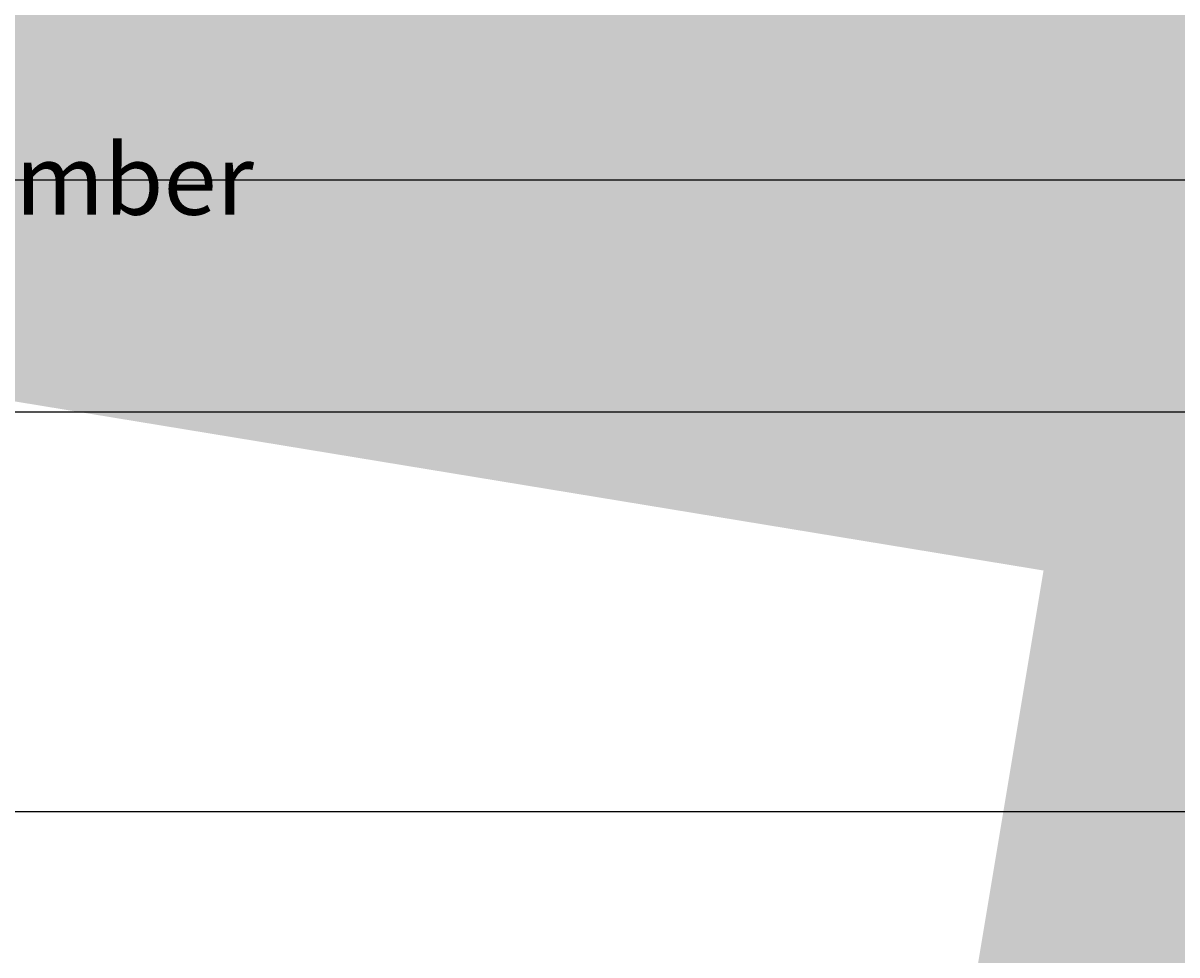
# Model space of a CAD drawing. Units: millimetres. Extents: x -22994 to 29398, y -19990 to 20176.
# Tile 56 of 135: x 247 to 296, y 25 to 65. Entities that reach past the tile are written whole.
import ezdxf
from ezdxf import colors
from ezdxf.entities.mleader import LeaderData, LeaderLine
from ezdxf.math import Vec2, Vec3

# ---------------------------------------------------------------- set-up
doc = ezdxf.new("R2010")
doc.units = ezdxf.units.MM
doc.header["$MEASUREMENT"] = 0
doc.layers.add('M-ANNO-TEXT', color=7, linetype='Continuous', lineweight=25)
doc.layers.add('M-DIMS', color=2, linetype='Continuous', lineweight=18)
doc.styles.get("Standard").update_dxf_attribs({"font": 'arial.ttf'})
doc.dimstyles.get("Standard").update_dxf_attribs({"dimtxt": 0.18, "dimasz": 10000, "dimexe": 0.18, "dimexo": 0.0625, "dimgap": 0.09, "dimtad": 0, "dimtih": 1, "dimtoh": 1, "dimdec": 0, "dimzin": 0, "dimdsep": 46, "dimtxsty": 'Standard', "dimcen": 0.09, "dimadec": 0, "dimazin": 0, "dimtfac": 1, "dimtdec": 0, "dimtofl": 0, "dimtmove": 0, "dimatfit": 3, "dimfxl": 1, "dimtolj": 1, "dimtzin": 0, "dimlwd": 30, "dimarcsym": 0})

# ---------------------------------------------------------------- blocks, each defined once
blk = doc.blocks.new('*D2')
at = {"layer": 'Defpoints', "color": 0, "transparency": 16777216}
for p in [(6.677, 10.271), (290.852, 10.271), (290.852, -5.079)]:
    blk.add_point(p, dxfattribs=at)
at = {"layer": 'M-DIMS', "color": 0, "lineweight": -2, "transparency": 16777216}
for p, q in [((6.677, 10.209), (6.677, -5.259)), ((290.852, 10.209), (290.852, -5.259))]:
    blk.add_line(p, q, dxfattribs=at)
at = {"layer": 'M-DIMS', "color": 0, "lineweight": 30, "transparency": 16777216}
for p, q in [((-9993.323, -5.079), (-19993.323, -5.079)), ((10290.852, -5.079), (20290.852, -5.079))]:
    blk.add_line(p, q, dxfattribs=at)
at = {"layer": 'M-DIMS', "color": 0, "transparency": 16777216}
for points in [[(-9993.323, 1661.588), (-9993.323, -1671.745), (6.677, -5.079)], [(10290.852, 1661.588), (10290.852, -1671.745), (290.852, -5.079)]]:
    blk.add_solid(points, dxfattribs=at)
at = {"layer": 'M-DIMS', "color": 0, "transparency": 16777216, "insert": (148.765, -5.079), "char_height": 0.18, "attachment_point": 5}
blk.add_mtext('\\A1;284.2', dxfattribs=at)
blk = doc.blocks.new('*D3')
at = {"layer": 'Defpoints', "color": 0, "transparency": 16777216}
for p in [(110.265, 204.165), (110.265, 176.366), (95.833, 127.967)]:
    blk.add_point(p, dxfattribs=at)
at = {"layer": 'M-DIMS', "color": 0, "lineweight": -2, "transparency": 16777216}
for p, q in [((95.833, 128.03), (95.833, 204.345)), ((110.265, 176.429), (110.265, 204.345))]:
    blk.add_line(p, q, dxfattribs=at)
at = {"layer": 'M-DIMS', "color": 0, "lineweight": 30, "transparency": 16777216}
for p, q in [((-9904.167, 204.165), (-19904.167, 204.165)), ((10110.265, 204.165), (20110.265, 204.165))]:
    blk.add_line(p, q, dxfattribs=at)
at = {"layer": 'M-DIMS', "color": 0, "transparency": 16777216}
for points in [[(-9904.167, 1870.832), (-9904.167, -1462.501), (95.833, 204.165)], [(10110.265, 1870.832), (10110.265, -1462.501), (110.265, 204.165)]]:
    blk.add_solid(points, dxfattribs=at)
at = {"layer": 'M-DIMS', "color": 0, "transparency": 16777216, "insert": (103.049, 204.165), "char_height": 0.18, "attachment_point": 5}
blk.add_mtext('\\A1;14.432', dxfattribs=at)
blk = doc.blocks.new('*D4')
at = {"layer": 'Defpoints', "color": 0, "transparency": 16777216}
for p in [(116.265, 204.165), (110.265, 176.366), (116.265, 176.366)]:
    blk.add_point(p, dxfattribs=at)
at = {"layer": 'M-DIMS', "color": 0, "lineweight": -2, "transparency": 16777216}
for p, q in [((110.265, 176.429), (110.265, 204.345)), ((116.265, 176.429), (116.265, 204.345))]:
    blk.add_line(p, q, dxfattribs=at)
at = {"layer": 'M-DIMS', "color": 0, "lineweight": 30, "transparency": 16777216}
for p, q in [((-9889.735, 204.165), (-19889.735, 204.165)), ((10116.265, 204.165), (20116.265, 204.165))]:
    blk.add_line(p, q, dxfattribs=at)
at = {"layer": 'M-DIMS', "color": 0, "transparency": 16777216}
for points in [[(-9889.735, 1870.832), (-9889.735, -1462.501), (110.265, 204.165)], [(10116.265, 1870.832), (10116.265, -1462.501), (116.265, 204.165)]]:
    blk.add_solid(points, dxfattribs=at)
at = {"layer": 'M-DIMS', "color": 0, "transparency": 16777216, "insert": (113.265, 204.165), "char_height": 0.18, "attachment_point": 5}
blk.add_mtext('\\A1;6', dxfattribs=at)
blk = doc.blocks.new('*D5')
at = {"layer": 'Defpoints', "color": 0, "transparency": 16777216}
for p in [(181.265, 204.165), (116.265, 176.366), (181.265, 176.366)]:
    blk.add_point(p, dxfattribs=at)
at = {"layer": 'M-DIMS', "color": 0, "lineweight": -2, "transparency": 16777216}
for p, q in [((116.265, 176.429), (116.265, 204.345)), ((181.265, 176.429), (181.265, 204.345))]:
    blk.add_line(p, q, dxfattribs=at)
at = {"layer": 'M-DIMS', "color": 0, "lineweight": 30, "transparency": 16777216}
for p, q in [((-9883.735, 204.165), (-19883.735, 204.165)), ((10181.265, 204.165), (20181.265, 204.165))]:
    blk.add_line(p, q, dxfattribs=at)
at = {"layer": 'M-DIMS', "color": 0, "transparency": 16777216}
for points in [[(-9883.735, 1870.832), (-9883.735, -1462.501), (116.265, 204.165)], [(10181.265, 1870.832), (10181.265, -1462.501), (181.265, 204.165)]]:
    blk.add_solid(points, dxfattribs=at)
at = {"layer": 'M-DIMS', "color": 0, "transparency": 16777216, "insert": (148.765, 204.165), "char_height": 0.18, "attachment_point": 5}
blk.add_mtext('\\A1;65', dxfattribs=at)
blk = doc.blocks.new('*D6')
at = {"layer": 'Defpoints', "color": 0, "transparency": 16777216}
for p in [(187.265, 204.165), (181.265, 176.366), (187.265, 176.366)]:
    blk.add_point(p, dxfattribs=at)
at = {"layer": 'M-DIMS', "color": 0, "lineweight": -2, "transparency": 16777216}
for p, q in [((181.265, 176.429), (181.265, 204.345)), ((187.265, 176.429), (187.265, 204.345))]:
    blk.add_line(p, q, dxfattribs=at)
at = {"layer": 'M-DIMS', "color": 0, "lineweight": 30, "transparency": 16777216}
for p, q in [((-9818.735, 204.165), (-19818.735, 204.165)), ((10187.265, 204.165), (20187.265, 204.165))]:
    blk.add_line(p, q, dxfattribs=at)
at = {"layer": 'M-DIMS', "color": 0, "transparency": 16777216}
for points in [[(-9818.735, 1870.832), (-9818.735, -1462.501), (181.265, 204.165)], [(10187.265, 1870.832), (10187.265, -1462.501), (187.265, 204.165)]]:
    blk.add_solid(points, dxfattribs=at)
at = {"layer": 'M-DIMS', "color": 0, "transparency": 16777216, "insert": (184.265, 204.165), "char_height": 0.18, "attachment_point": 5}
blk.add_mtext('\\A1;6', dxfattribs=at)
blk = doc.blocks.new('*D7')
at = {"layer": 'Defpoints', "color": 0, "transparency": 16777216}
for p in [(201.697, 204.165), (187.265, 176.366), (201.697, 127.967)]:
    blk.add_point(p, dxfattribs=at)
at = {"layer": 'M-DIMS', "color": 0, "lineweight": -2, "transparency": 16777216}
for p, q in [((187.265, 176.429), (187.265, 204.345)), ((201.697, 128.03), (201.697, 204.345))]:
    blk.add_line(p, q, dxfattribs=at)
at = {"layer": 'M-DIMS', "color": 0, "lineweight": 30, "transparency": 16777216}
for p, q in [((-9812.735, 204.165), (-19812.735, 204.165)), ((10201.697, 204.165), (20201.697, 204.165))]:
    blk.add_line(p, q, dxfattribs=at)
at = {"layer": 'M-DIMS', "color": 0, "transparency": 16777216}
for points in [[(-9812.735, 1870.832), (-9812.735, -1462.501), (187.265, 204.165)], [(10201.697, 1870.832), (10201.697, -1462.501), (201.697, 204.165)]]:
    blk.add_solid(points, dxfattribs=at)
at = {"layer": 'M-DIMS', "color": 0, "transparency": 16777216, "insert": (194.481, 204.165), "char_height": 0.18, "attachment_point": 5}
blk.add_mtext('\\A1;14.432', dxfattribs=at)
blk = doc.blocks.new('*D8')
at = {"layer": 'Defpoints', "color": 0, "transparency": 16777216}
for p in [(227.648, 204.165), (227.648, 146.73), (201.697, 127.967)]:
    blk.add_point(p, dxfattribs=at)
at = {"layer": 'M-DIMS', "color": 0, "lineweight": -2, "transparency": 16777216}
for p, q in [((201.697, 128.03), (201.697, 204.345)), ((227.648, 146.792), (227.648, 204.345))]:
    blk.add_line(p, q, dxfattribs=at)
at = {"layer": 'M-DIMS', "color": 0, "lineweight": 30, "transparency": 16777216}
for p, q in [((-9798.303, 204.165), (-19798.303, 204.165)), ((10227.648, 204.165), (20227.648, 204.165))]:
    blk.add_line(p, q, dxfattribs=at)
at = {"layer": 'M-DIMS', "color": 0, "transparency": 16777216}
for points in [[(-9798.303, 1870.832), (-9798.303, -1462.501), (201.697, 204.165)], [(10227.648, 1870.832), (10227.648, -1462.501), (227.648, 204.165)]]:
    blk.add_solid(points, dxfattribs=at)
at = {"layer": 'M-DIMS', "color": 0, "transparency": 16777216, "insert": (214.673, 204.165), "char_height": 0.18, "attachment_point": 5}
blk.add_mtext('\\A1;25.95', dxfattribs=at)
blk = doc.blocks.new('*D9')
at = {"layer": 'Defpoints', "color": 0, "transparency": 16777216}
for p in [(187.265, 176.366), (306.202, 176.366), (290.852, 10.271)]:
    blk.add_point(p, dxfattribs=at)
at = {"layer": 'M-DIMS', "color": 0, "lineweight": 30, "transparency": 16777216}
for p, q in [((306.202, 10176.366), (306.202, 20176.366)), ((306.202, -9989.729), (306.202, -19989.729))]:
    blk.add_line(p, q, dxfattribs=at)
at = {"layer": 'M-DIMS', "color": 0, "lineweight": -2, "transparency": 16777216}
for p, q in [((187.327, 176.366), (306.382, 176.366)), ((290.915, 10.271), (306.382, 10.271))]:
    blk.add_line(p, q, dxfattribs=at)
at = {"layer": 'M-DIMS', "color": 0, "transparency": 16777216}
for points in [[(-1360.465, 10176.366), (1972.869, 10176.366), (306.202, 176.366)], [(-1360.465, -9989.729), (1972.869, -9989.729), (306.202, 10.271)]]:
    blk.add_solid(points, dxfattribs=at)
at = {"layer": 'M-DIMS', "color": 0, "transparency": 16777216, "insert": (306.202, 93.319), "char_height": 0.18, "attachment_point": 5}
blk.add_mtext('\\A1;166.1', dxfattribs=at)
blk = doc.blocks.new('*D10')
at = {"layer": 'Defpoints', "color": 0, "transparency": 16777216}
for p in [(125.65, 136.071), (133.346, 136.071), (133.346, -5.079)]:
    blk.add_point(p, dxfattribs=at)
at = {"layer": 'M-DIMS', "color": 0, "lineweight": -2, "transparency": 16777216}
for p, q in [((125.65, 136.009), (125.65, -5.259)), ((133.346, 136.009), (133.346, -5.259))]:
    blk.add_line(p, q, dxfattribs=at)
at = {"layer": 'M-DIMS', "color": 0, "lineweight": 30, "transparency": 16777216}
for p, q in [((-9874.35, -5.079), (-19874.35, -5.079)), ((10133.346, -5.079), (20133.346, -5.079))]:
    blk.add_line(p, q, dxfattribs=at)
at = {"layer": 'M-DIMS', "color": 0, "transparency": 16777216}
for points in [[(-9874.35, 1661.588), (-9874.35, -1671.745), (125.65, -5.079)], [(10133.346, 1661.588), (10133.346, -1671.745), (133.346, -5.079)]]:
    blk.add_solid(points, dxfattribs=at)
at = {"layer": 'M-DIMS', "color": 0, "transparency": 16777216, "insert": (129.498, -5.079), "char_height": 0.18, "attachment_point": 5}
blk.add_mtext('\\A1;7.696', dxfattribs=at)
blk = doc.blocks.new('*D11')
at = {"layer": 'Defpoints', "color": 0, "transparency": 16777216}
for p in [(133.346, 136.071), (135.65, 136.071), (135.65, -5.079)]:
    blk.add_point(p, dxfattribs=at)
at = {"layer": 'M-DIMS', "color": 0, "lineweight": -2, "transparency": 16777216}
for p, q in [((133.346, 136.009), (133.346, -5.259)), ((135.65, 136.009), (135.65, -5.259))]:
    blk.add_line(p, q, dxfattribs=at)
at = {"layer": 'M-DIMS', "color": 0, "lineweight": 30, "transparency": 16777216}
for p, q in [((-9866.654, -5.079), (-19866.654, -5.079)), ((10135.65, -5.079), (20135.65, -5.079))]:
    blk.add_line(p, q, dxfattribs=at)
at = {"layer": 'M-DIMS', "color": 0, "transparency": 16777216}
for points in [[(-9866.654, 1661.588), (-9866.654, -1671.745), (133.346, -5.079)], [(10135.65, 1661.588), (10135.65, -1671.745), (135.65, -5.079)]]:
    blk.add_solid(points, dxfattribs=at)
at = {"layer": 'M-DIMS', "color": 0, "transparency": 16777216, "insert": (134.498, -5.079), "char_height": 0.18, "attachment_point": 5}
blk.add_mtext('\\A1;2.304', dxfattribs=at)
blk = doc.blocks.new('*D12')
at = {"layer": 'Defpoints', "color": 0, "transparency": 16777216}
for p in [(135.65, 136.071), (145.65, 136.071), (145.65, -5.079)]:
    blk.add_point(p, dxfattribs=at)
at = {"layer": 'M-DIMS', "color": 0, "lineweight": -2, "transparency": 16777216}
for p, q in [((135.65, 136.009), (135.65, -5.259)), ((145.65, 136.009), (145.65, -5.259))]:
    blk.add_line(p, q, dxfattribs=at)
at = {"layer": 'M-DIMS', "color": 0, "lineweight": 30, "transparency": 16777216}
for p, q in [((-9864.35, -5.079), (-19864.35, -5.079)), ((10145.65, -5.079), (20145.65, -5.079))]:
    blk.add_line(p, q, dxfattribs=at)
at = {"layer": 'M-DIMS', "color": 0, "transparency": 16777216}
for points in [[(-9864.35, 1661.588), (-9864.35, -1671.745), (135.65, -5.079)], [(10145.65, 1661.588), (10145.65, -1671.745), (145.65, -5.079)]]:
    blk.add_solid(points, dxfattribs=at)
at = {"layer": 'M-DIMS', "color": 0, "transparency": 16777216, "insert": (140.65, -5.079), "char_height": 0.18, "attachment_point": 5}
blk.add_mtext('\\A1;10', dxfattribs=at)
blk = doc.blocks.new('*D13')
at = {"layer": 'Defpoints', "color": 0, "transparency": 16777216}
for p in [(145.65, 136.071), (155.65, 136.071), (155.65, -5.079)]:
    blk.add_point(p, dxfattribs=at)
at = {"layer": 'M-DIMS', "color": 0, "lineweight": -2, "transparency": 16777216}
for p, q in [((145.65, 136.009), (145.65, -5.259)), ((155.65, 136.009), (155.65, -5.259))]:
    blk.add_line(p, q, dxfattribs=at)
at = {"layer": 'M-DIMS', "color": 0, "lineweight": 30, "transparency": 16777216}
for p, q in [((-9854.35, -5.079), (-19854.35, -5.079)), ((10155.65, -5.079), (20155.65, -5.079))]:
    blk.add_line(p, q, dxfattribs=at)
at = {"layer": 'M-DIMS', "color": 0, "transparency": 16777216}
for points in [[(-9854.35, 1661.588), (-9854.35, -1671.745), (145.65, -5.079)], [(10155.65, 1661.588), (10155.65, -1671.745), (155.65, -5.079)]]:
    blk.add_solid(points, dxfattribs=at)
at = {"layer": 'M-DIMS', "color": 0, "transparency": 16777216, "insert": (150.65, -5.079), "char_height": 0.18, "attachment_point": 5}
blk.add_mtext('\\A1;10', dxfattribs=at)
blk = doc.blocks.new('*D14')
at = {"layer": 'Defpoints', "color": 0, "transparency": 16777216}
for p in [(155.65, 136.071), (165.65, 136.071), (165.65, -5.079)]:
    blk.add_point(p, dxfattribs=at)
at = {"layer": 'M-DIMS', "color": 0, "lineweight": -2, "transparency": 16777216}
for p, q in [((155.65, 136.009), (155.65, -5.259)), ((165.65, 136.009), (165.65, -5.259))]:
    blk.add_line(p, q, dxfattribs=at)
at = {"layer": 'M-DIMS', "color": 0, "lineweight": 30, "transparency": 16777216}
for p, q in [((-9844.35, -5.079), (-19844.35, -5.079)), ((10165.65, -5.079), (20165.65, -5.079))]:
    blk.add_line(p, q, dxfattribs=at)
at = {"layer": 'M-DIMS', "color": 0, "transparency": 16777216}
for points in [[(-9844.35, 1661.588), (-9844.35, -1671.745), (155.65, -5.079)], [(10165.65, 1661.588), (10165.65, -1671.745), (165.65, -5.079)]]:
    blk.add_solid(points, dxfattribs=at)
at = {"layer": 'M-DIMS', "color": 0, "transparency": 16777216, "insert": (160.65, -5.079), "char_height": 0.18, "attachment_point": 5}
blk.add_mtext('\\A1;10', dxfattribs=at)
blk = doc.blocks.new('*D15')
at = {"layer": 'Defpoints', "color": 0, "transparency": 16777216}
for p in [(173.346, 154.788), (173.346, 136.071), (306.202, 136.071)]:
    blk.add_point(p, dxfattribs=at)
at = {"layer": 'M-DIMS', "color": 0, "lineweight": 30, "transparency": 16777216}
for p, q in [((306.202, 10154.788), (306.202, 20154.788)), ((306.202, -9863.929), (306.202, -19863.929))]:
    blk.add_line(p, q, dxfattribs=at)
at = {"layer": 'M-DIMS', "color": 0, "lineweight": -2, "transparency": 16777216}
for p, q in [((173.408, 154.788), (306.382, 154.788)), ((173.408, 136.071), (306.382, 136.071))]:
    blk.add_line(p, q, dxfattribs=at)
at = {"layer": 'M-DIMS', "color": 0, "transparency": 16777216}
for points in [[(-1360.465, 10154.788), (1972.869, 10154.788), (306.202, 154.788)], [(-1360.465, -9863.929), (1972.869, -9863.929), (306.202, 136.071)]]:
    blk.add_solid(points, dxfattribs=at)
at = {"layer": 'M-DIMS', "color": 0, "transparency": 16777216, "insert": (306.202, 145.43), "char_height": 0.18, "attachment_point": 5}
blk.add_mtext('\\A1;18.717', dxfattribs=at)
blk = doc.blocks.new('*D16')
at = {"layer": 'Defpoints', "color": 0, "transparency": 16777216}
for p in [(120.17, 204.165), (110.466, 48.035), (120.17, 48.035)]:
    blk.add_point(p, dxfattribs=at)
at = {"layer": 'M-DIMS', "color": 0, "lineweight": -2, "transparency": 16777216}
for p, q in [((110.466, 48.097), (110.466, 204.345)), ((120.17, 48.097), (120.17, 204.345))]:
    blk.add_line(p, q, dxfattribs=at)
at = {"layer": 'M-DIMS', "color": 0, "lineweight": 30, "transparency": 16777216}
for p, q in [((-9889.534, 204.165), (-19889.534, 204.165)), ((10120.17, 204.165), (20120.17, 204.165))]:
    blk.add_line(p, q, dxfattribs=at)
at = {"layer": 'M-DIMS', "color": 0, "transparency": 16777216}
for points in [[(-9889.534, 1870.832), (-9889.534, -1462.501), (110.466, 204.165)], [(10120.17, 1870.832), (10120.17, -1462.501), (120.17, 204.165)]]:
    blk.add_solid(points, dxfattribs=at)
at = {"layer": 'M-DIMS', "color": 0, "transparency": 16777216, "insert": (115.318, 204.165), "char_height": 0.18, "attachment_point": 5}
blk.add_mtext('\\A1;9.704', dxfattribs=at)
blk = doc.blocks.new('*D17')
at = {"layer": 'Defpoints', "color": 0, "transparency": 16777216}
for p in [(126.17, 204.165), (120.17, 48.035), (126.17, 48.035)]:
    blk.add_point(p, dxfattribs=at)
at = {"layer": 'M-DIMS', "color": 0, "lineweight": -2, "transparency": 16777216}
for p, q in [((120.17, 48.097), (120.17, 204.345)), ((126.17, 48.097), (126.17, 204.345))]:
    blk.add_line(p, q, dxfattribs=at)
at = {"layer": 'M-DIMS', "color": 0, "lineweight": 30, "transparency": 16777216}
for p, q in [((-9879.83, 204.165), (-19879.83, 204.165)), ((10126.17, 204.165), (20126.17, 204.165))]:
    blk.add_line(p, q, dxfattribs=at)
at = {"layer": 'M-DIMS', "color": 0, "transparency": 16777216}
for points in [[(-9879.83, 1870.832), (-9879.83, -1462.501), (120.17, 204.165)], [(10126.17, 1870.832), (10126.17, -1462.501), (126.17, 204.165)]]:
    blk.add_solid(points, dxfattribs=at)
at = {"layer": 'M-DIMS', "color": 0, "transparency": 16777216, "insert": (123.17, 204.165), "char_height": 0.18, "attachment_point": 5}
blk.add_mtext('\\A1;6', dxfattribs=at)
blk = doc.blocks.new('*D18')
at = {"layer": 'Defpoints', "color": 0, "transparency": 16777216}
for p in [(132.17, 204.165), (126.17, 48.035), (132.17, 48.035)]:
    blk.add_point(p, dxfattribs=at)
at = {"layer": 'M-DIMS', "color": 0, "lineweight": -2, "transparency": 16777216}
for p, q in [((126.17, 48.097), (126.17, 204.345)), ((132.17, 48.097), (132.17, 204.345))]:
    blk.add_line(p, q, dxfattribs=at)
at = {"layer": 'M-DIMS', "color": 0, "lineweight": 30, "transparency": 16777216}
for p, q in [((-9873.83, 204.165), (-19873.83, 204.165)), ((10132.17, 204.165), (20132.17, 204.165))]:
    blk.add_line(p, q, dxfattribs=at)
at = {"layer": 'M-DIMS', "color": 0, "transparency": 16777216}
for points in [[(-9873.83, 1870.832), (-9873.83, -1462.501), (126.17, 204.165)], [(10132.17, 1870.832), (10132.17, -1462.501), (132.17, 204.165)]]:
    blk.add_solid(points, dxfattribs=at)
at = {"layer": 'M-DIMS', "color": 0, "transparency": 16777216, "insert": (129.17, 204.165), "char_height": 0.18, "attachment_point": 5}
blk.add_mtext('\\A1;6', dxfattribs=at)
blk = doc.blocks.new('*D19')
at = {"layer": 'Defpoints', "color": 0, "transparency": 16777216}
for p in [(138.17, 204.165), (132.17, 48.035), (138.17, 48.035)]:
    blk.add_point(p, dxfattribs=at)
at = {"layer": 'M-DIMS', "color": 0, "lineweight": -2, "transparency": 16777216}
for p, q in [((132.17, 48.097), (132.17, 204.345)), ((138.17, 48.097), (138.17, 204.345))]:
    blk.add_line(p, q, dxfattribs=at)
at = {"layer": 'M-DIMS', "color": 0, "lineweight": 30, "transparency": 16777216}
for p, q in [((-9867.83, 204.165), (-19867.83, 204.165)), ((10138.17, 204.165), (20138.17, 204.165))]:
    blk.add_line(p, q, dxfattribs=at)
at = {"layer": 'M-DIMS', "color": 0, "transparency": 16777216}
for points in [[(-9867.83, 1870.832), (-9867.83, -1462.501), (132.17, 204.165)], [(10138.17, 1870.832), (10138.17, -1462.501), (138.17, 204.165)]]:
    blk.add_solid(points, dxfattribs=at)
at = {"layer": 'M-DIMS', "color": 0, "transparency": 16777216, "insert": (135.17, 204.165), "char_height": 0.18, "attachment_point": 5}
blk.add_mtext('\\A1;6', dxfattribs=at)
blk = doc.blocks.new('*D20')
at = {"layer": 'Defpoints', "color": 0, "transparency": 16777216}
for p in [(144.17, 204.165), (138.17, 48.035), (144.17, 48.035)]:
    blk.add_point(p, dxfattribs=at)
at = {"layer": 'M-DIMS', "color": 0, "lineweight": -2, "transparency": 16777216}
for p, q in [((138.17, 48.097), (138.17, 204.345)), ((144.17, 48.097), (144.17, 204.345))]:
    blk.add_line(p, q, dxfattribs=at)
at = {"layer": 'M-DIMS', "color": 0, "lineweight": 30, "transparency": 16777216}
for p, q in [((-9861.83, 204.165), (-19861.83, 204.165)), ((10144.17, 204.165), (20144.17, 204.165))]:
    blk.add_line(p, q, dxfattribs=at)
at = {"layer": 'M-DIMS', "color": 0, "transparency": 16777216}
for points in [[(-9861.83, 1870.832), (-9861.83, -1462.501), (138.17, 204.165)], [(10144.17, 1870.832), (10144.17, -1462.501), (144.17, 204.165)]]:
    blk.add_solid(points, dxfattribs=at)
at = {"layer": 'M-DIMS', "color": 0, "transparency": 16777216, "insert": (141.17, 204.165), "char_height": 0.18, "attachment_point": 5}
blk.add_mtext('\\A1;6', dxfattribs=at)
blk = doc.blocks.new('*D21')
at = {"layer": 'Defpoints', "color": 0, "transparency": 16777216}
for p in [(149.116, 204.165), (144.17, 48.035), (149.116, 48.035)]:
    blk.add_point(p, dxfattribs=at)
at = {"layer": 'M-DIMS', "color": 0, "lineweight": -2, "transparency": 16777216}
for p, q in [((144.17, 48.097), (144.17, 204.345)), ((149.116, 48.097), (149.116, 204.345))]:
    blk.add_line(p, q, dxfattribs=at)
at = {"layer": 'M-DIMS', "color": 0, "lineweight": 30, "transparency": 16777216}
for p, q in [((-9855.83, 204.165), (-19855.83, 204.165)), ((10149.116, 204.165), (20149.116, 204.165))]:
    blk.add_line(p, q, dxfattribs=at)
at = {"layer": 'M-DIMS', "color": 0, "transparency": 16777216}
for points in [[(-9855.83, 1870.832), (-9855.83, -1462.501), (144.17, 204.165)], [(10149.116, 1870.832), (10149.116, -1462.501), (149.116, 204.165)]]:
    blk.add_solid(points, dxfattribs=at)
at = {"layer": 'M-DIMS', "color": 0, "transparency": 16777216, "insert": (146.643, 204.165), "char_height": 0.18, "attachment_point": 5}
blk.add_mtext('\\A1;4.945', dxfattribs=at)
blk = doc.blocks.new('*D22')
at = {"layer": 'Defpoints', "color": 0, "transparency": 16777216}
for p in [(149.116, 30.99), (155.116, 30.99), (155.116, -5.079)]:
    blk.add_point(p, dxfattribs=at)
at = {"layer": 'M-DIMS', "color": 0, "lineweight": -2, "transparency": 16777216}
for p, q in [((149.116, 30.927), (149.116, -5.259)), ((155.116, 30.927), (155.116, -5.259))]:
    blk.add_line(p, q, dxfattribs=at)
at = {"layer": 'M-DIMS', "color": 0, "lineweight": 30, "transparency": 16777216}
for p, q in [((-9850.884, -5.079), (-19850.884, -5.079)), ((10155.116, -5.079), (20155.116, -5.079))]:
    blk.add_line(p, q, dxfattribs=at)
at = {"layer": 'M-DIMS', "color": 0, "transparency": 16777216}
for points in [[(-9850.884, 1661.588), (-9850.884, -1671.745), (149.116, -5.079)], [(10155.116, 1661.588), (10155.116, -1671.745), (155.116, -5.079)]]:
    blk.add_solid(points, dxfattribs=at)
at = {"layer": 'M-DIMS', "color": 0, "transparency": 16777216, "insert": (152.116, -5.079), "char_height": 0.18, "attachment_point": 5}
blk.add_mtext('\\A1;6', dxfattribs=at)
blk = doc.blocks.new('*D23')
at = {"layer": 'Defpoints', "color": 0, "transparency": 16777216}
for p in [(155.116, 30.99), (161.116, 30.99), (161.116, -5.079)]:
    blk.add_point(p, dxfattribs=at)
at = {"layer": 'M-DIMS', "color": 0, "lineweight": -2, "transparency": 16777216}
for p, q in [((155.116, 30.927), (155.116, -5.259)), ((161.116, 30.927), (161.116, -5.259))]:
    blk.add_line(p, q, dxfattribs=at)
at = {"layer": 'M-DIMS', "color": 0, "lineweight": 30, "transparency": 16777216}
for p, q in [((-9844.884, -5.079), (-19844.884, -5.079)), ((10161.116, -5.079), (20161.116, -5.079))]:
    blk.add_line(p, q, dxfattribs=at)
at = {"layer": 'M-DIMS', "color": 0, "transparency": 16777216}
for points in [[(-9844.884, 1661.588), (-9844.884, -1671.745), (155.116, -5.079)], [(10161.116, 1661.588), (10161.116, -1671.745), (161.116, -5.079)]]:
    blk.add_solid(points, dxfattribs=at)
at = {"layer": 'M-DIMS', "color": 0, "transparency": 16777216, "insert": (158.116, -5.079), "char_height": 0.18, "attachment_point": 5}
blk.add_mtext('\\A1;6', dxfattribs=at)
blk = doc.blocks.new('*D24')
at = {"layer": 'Defpoints', "color": 0, "transparency": 16777216}
for p in [(161.116, 30.99), (166.439, 30.99), (166.439, -5.079)]:
    blk.add_point(p, dxfattribs=at)
at = {"layer": 'M-DIMS', "color": 0, "lineweight": -2, "transparency": 16777216}
for p, q in [((161.116, 30.927), (161.116, -5.259)), ((166.439, 30.927), (166.439, -5.259))]:
    blk.add_line(p, q, dxfattribs=at)
at = {"layer": 'M-DIMS', "color": 0, "lineweight": 30, "transparency": 16777216}
for p, q in [((-9838.884, -5.079), (-19838.884, -5.079)), ((10166.439, -5.079), (20166.439, -5.079))]:
    blk.add_line(p, q, dxfattribs=at)
at = {"layer": 'M-DIMS', "color": 0, "transparency": 16777216}
for points in [[(-9838.884, 1661.588), (-9838.884, -1671.745), (161.116, -5.079)], [(10166.439, 1661.588), (10166.439, -1671.745), (166.439, -5.079)]]:
    blk.add_solid(points, dxfattribs=at)
at = {"layer": 'M-DIMS', "color": 0, "transparency": 16777216, "insert": (163.777, -5.079), "char_height": 0.18, "attachment_point": 5}
blk.add_mtext('\\A1;5.323', dxfattribs=at)
blk = doc.blocks.new('*D25')
at = {"layer": 'Defpoints', "color": 0, "transparency": 16777216}
for p in [(166.439, 30.99), (172.439, 30.99), (172.439, -5.079)]:
    blk.add_point(p, dxfattribs=at)
at = {"layer": 'M-DIMS', "color": 0, "lineweight": -2, "transparency": 16777216}
for p, q in [((166.439, 30.927), (166.439, -5.259)), ((172.439, 30.927), (172.439, -5.259))]:
    blk.add_line(p, q, dxfattribs=at)
at = {"layer": 'M-DIMS', "color": 0, "lineweight": 30, "transparency": 16777216}
for p, q in [((-9833.561, -5.079), (-19833.561, -5.079)), ((10172.439, -5.079), (20172.439, -5.079))]:
    blk.add_line(p, q, dxfattribs=at)
at = {"layer": 'M-DIMS', "color": 0, "transparency": 16777216}
for points in [[(-9833.561, 1661.588), (-9833.561, -1671.745), (166.439, -5.079)], [(10172.439, 1661.588), (10172.439, -1671.745), (172.439, -5.079)]]:
    blk.add_solid(points, dxfattribs=at)
at = {"layer": 'M-DIMS', "color": 0, "transparency": 16777216, "insert": (169.439, -5.079), "char_height": 0.18, "attachment_point": 5}
blk.add_mtext('\\A1;6', dxfattribs=at)
blk = doc.blocks.new('*D26')
at = {"layer": 'Defpoints', "color": 0, "transparency": 16777216}
for p in [(172.439, 30.99), (178.439, 30.99), (178.439, -5.079)]:
    blk.add_point(p, dxfattribs=at)
at = {"layer": 'M-DIMS', "color": 0, "lineweight": -2, "transparency": 16777216}
for p, q in [((172.439, 30.927), (172.439, -5.259)), ((178.439, 30.927), (178.439, -5.259))]:
    blk.add_line(p, q, dxfattribs=at)
at = {"layer": 'M-DIMS', "color": 0, "lineweight": 30, "transparency": 16777216}
for p, q in [((-9827.561, -5.079), (-19827.561, -5.079)), ((10178.439, -5.079), (20178.439, -5.079))]:
    blk.add_line(p, q, dxfattribs=at)
at = {"layer": 'M-DIMS', "color": 0, "transparency": 16777216}
for points in [[(-9827.561, 1661.588), (-9827.561, -1671.745), (172.439, -5.079)], [(10178.439, 1661.588), (10178.439, -1671.745), (178.439, -5.079)]]:
    blk.add_solid(points, dxfattribs=at)
at = {"layer": 'M-DIMS', "color": 0, "transparency": 16777216, "insert": (175.439, -5.079), "char_height": 0.18, "attachment_point": 5}
blk.add_mtext('\\A1;6', dxfattribs=at)
blk = doc.blocks.new('*D27')
at = {"layer": 'Defpoints', "color": 0, "transparency": 16777216}
for p in [(178.439, 30.99), (188.117, 30.99), (188.117, -5.079)]:
    blk.add_point(p, dxfattribs=at)
at = {"layer": 'M-DIMS', "color": 0, "lineweight": -2, "transparency": 16777216}
for p, q in [((178.439, 30.927), (178.439, -5.259)), ((188.117, 30.927), (188.117, -5.259))]:
    blk.add_line(p, q, dxfattribs=at)
at = {"layer": 'M-DIMS', "color": 0, "lineweight": 30, "transparency": 16777216}
for p, q in [((-9821.561, -5.079), (-19821.561, -5.079)), ((10188.117, -5.079), (20188.117, -5.079))]:
    blk.add_line(p, q, dxfattribs=at)
at = {"layer": 'M-DIMS', "color": 0, "transparency": 16777216}
for points in [[(-9821.561, 1661.588), (-9821.561, -1671.745), (178.439, -5.079)], [(10188.117, 1661.588), (10188.117, -1671.745), (188.117, -5.079)]]:
    blk.add_solid(points, dxfattribs=at)
at = {"layer": 'M-DIMS', "color": 0, "transparency": 16777216, "insert": (183.278, -5.079), "char_height": 0.18, "attachment_point": 5}
blk.add_mtext('\\A1;9.679', dxfattribs=at)
blk = doc.blocks.new('*D28')
at = {"layer": 'Defpoints', "color": 0, "transparency": 16777216}
for p in [(188.117, 48.035), (306.202, 48.035), (188.117, 30.99)]:
    blk.add_point(p, dxfattribs=at)
at = {"layer": 'M-DIMS', "color": 0, "lineweight": 30, "transparency": 16777216}
for p, q in [((306.202, 10048.035), (306.202, 20048.035)), ((306.202, -9969.01), (306.202, -19969.01))]:
    blk.add_line(p, q, dxfattribs=at)
at = {"layer": 'M-DIMS', "color": 0, "lineweight": -2, "transparency": 16777216}
for p, q in [((188.18, 48.035), (306.382, 48.035)), ((188.18, 30.99), (306.382, 30.99))]:
    blk.add_line(p, q, dxfattribs=at)
at = {"layer": 'M-DIMS', "color": 0, "transparency": 16777216}
for points in [[(-1360.465, 10048.035), (1972.869, 10048.035), (306.202, 48.035)], [(-1360.465, -9969.01), (1972.869, -9969.01), (306.202, 30.99)]]:
    blk.add_solid(points, dxfattribs=at)
at = {"layer": 'M-DIMS', "color": 0, "transparency": 16777216, "insert": (306.202, 39.512), "char_height": 0.18, "attachment_point": 5}
blk.add_mtext('\\A1;17.045', dxfattribs=at)
blk = doc.blocks.new('*D29')
at = {"layer": 'Defpoints', "color": 0, "transparency": 16777216}
for p in [(36.801, 80.045), (64.03, 80.045)]:
    blk.add_point(p, dxfattribs=at)
at = {"layer": 'M-DIMS', "color": 0, "lineweight": -2, "transparency": 16777216}
for p, q in [((50.325, 80.045), (50.505, 80.045)), ((50.415, 79.955), (50.415, 80.135))]:
    blk.add_line(p, q, dxfattribs=at)
at = {"layer": 'M-DIMS', "color": 0, "lineweight": 30, "transparency": 16777216}
blk.add_line((20064.03, 80.03), (10064.03, 80.038), dxfattribs=at)
at = {"layer": 'M-DIMS', "color": 0, "transparency": 16777216}
blk.add_solid([(10064.031, 1746.704), (10064.028, -1586.629), (64.03, 80.045)], dxfattribs=at)
at = {"layer": 'M-DIMS', "color": 0, "transparency": 16777216, "insert": (20064.521, 80.03), "char_height": 0.18, "attachment_point": 5}
blk.add_mtext('\\A1;∅27.23', dxfattribs=at)
blk = doc.blocks.new('*D30')
at = {"layer": 'Defpoints', "color": 0, "transparency": 16777216}
for p in [(216.315, 146.729), (238.982, 146.73)]:
    blk.add_point(p, dxfattribs=at)
at = {"layer": 'M-DIMS', "color": 0, "lineweight": 30, "transparency": 16777216}
blk.add_line((20238.982, 147.496), (10238.982, 147.113), dxfattribs=at)
at = {"layer": 'M-DIMS', "color": 0, "lineweight": -2, "transparency": 16777216}
for p, q in [((227.558, 146.73), (227.738, 146.73)), ((227.648, 146.64), (227.648, 146.82))]:
    blk.add_line(p, q, dxfattribs=at)
at = {"layer": 'M-DIMS', "color": 0, "transparency": 16777216}
blk.add_solid([(10238.918, 1813.78), (10239.046, -1519.554), (238.982, 146.73)], dxfattribs=at)
at = {"layer": 'M-DIMS', "color": 0, "transparency": 16777216, "insert": (20239.544, 147.496), "char_height": 0.18, "attachment_point": 5}
blk.add_mtext('\\A1;∅22.667', dxfattribs=at)
blk = doc.blocks.new('*D31')
at = {"layer": 'Defpoints', "color": 0, "transparency": 16777216}
for p in [(223.164, 146.729), (232.133, 146.73)]:
    blk.add_point(p, dxfattribs=at)
at = {"layer": 'M-DIMS', "color": 0, "lineweight": 30, "transparency": 16777216}
blk.add_line((20232.133, 148.666), (10232.133, 147.698), dxfattribs=at)
at = {"layer": 'M-DIMS', "color": 0, "lineweight": -2, "transparency": 16777216}
for p, q in [((227.558, 146.73), (227.738, 146.73)), ((227.648, 146.64), (227.648, 146.82))]:
    blk.add_line(p, q, dxfattribs=at)
at = {"layer": 'M-DIMS', "color": 0, "transparency": 16777216}
blk.add_solid([(10231.971, 1814.364), (10232.294, -1518.969), (232.133, 146.73)], dxfattribs=at)
at = {"layer": 'M-DIMS', "color": 0, "transparency": 16777216, "insert": (20232.625, 148.666), "char_height": 0.18, "attachment_point": 5}
blk.add_mtext('\\A1;∅8.969', dxfattribs=at)
blk = doc.blocks.new('*D33')
at = {"layer": 'Defpoints', "color": 0, "transparency": 16777216}
for p in [(229.561, 154.377), (232.997, 153.351)]:
    blk.add_point(p, dxfattribs=at)
at = {"layer": 'M-DIMS', "color": 0, "lineweight": -2, "transparency": 16777216}
for p, q in [((229.471, 154.377), (229.651, 154.377)), ((229.561, 154.287), (229.561, 154.467))]:
    blk.add_line(p, q, dxfattribs=at)
at = {"layer": 'M-DIMS', "color": 0, "lineweight": 30, "transparency": 16777216}
for p, q in [((19396.339, -5570.838), (9814.668, -2708.743)), ((29396.339, -5570.838), (19396.339, -5570.838))]:
    blk.add_line(p, q, dxfattribs=at)
at = {"layer": 'M-DIMS', "color": 0, "transparency": 16777216}
blk.add_solid([(10291.684, -1111.798), (9337.652, -4305.689), (232.997, 153.351)], dxfattribs=at)
at = {"layer": 'M-DIMS', "color": 0, "transparency": 16777216, "insert": (29397.012, -5570.838), "char_height": 0.18, "attachment_point": 5}
blk.add_mtext('\\A1;6X R3.586', dxfattribs=at)
blk = doc.blocks.new('*D36')
at = {"layer": 'Defpoints', "color": 0, "transparency": 16777216}
for p in [(46.39, 31.303), (46.387, 26.593)]:
    blk.add_point(p, dxfattribs=at)
at = {"layer": 'M-DIMS', "color": 0, "lineweight": 30, "transparency": 16777216}
for p, q in [((57.15, 20031.301), (51.77, 10031.302)), ((10057.15, 20031.301), (57.15, 20031.301))]:
    blk.add_line(p, q, dxfattribs=at)
at = {"layer": 'M-DIMS', "color": 0, "lineweight": -2, "transparency": 16777216}
for p, q in [((46.389, 28.858), (46.389, 29.038)), ((46.299, 28.948), (46.479, 28.948))]:
    blk.add_line(p, q, dxfattribs=at)
at = {"layer": 'M-DIMS', "color": 0, "transparency": 16777216}
blk.add_solid([(-1614.896, 10032.199), (1718.436, 10030.405), (46.39, 31.303)], dxfattribs=at)
at = {"layer": 'M-DIMS', "color": 0, "transparency": 16777216, "insert": (10057.554, 20031.301), "char_height": 0.18, "attachment_point": 5}
blk.add_mtext('\\A1;∅4.71', dxfattribs=at)

msp = doc.modelspace()

# ---------------------------------------------------------------- dimensions: what is measured, and where the dimension line sits
at = {"layer": 'M-DIMS'}
for base, p1, p2, override, picture, middle in [((306.202, 176.3662), (290.852, 10.2713), (187.2647, 176.3662), {"dimdec": 1, "dimlfac": 1, "dimrnd": 0, "dimzin": 0, "dimdsep": 46, "dimlunit": 2}, '*D9', (306.202, 93.3187)), ((306.202, 136.0713), (173.3459, 154.788), (173.3459, 136.0713), {"dimdec": 3, "dimlfac": 1, "dimrnd": 0, "dimzin": 0, "dimdsep": 46, "dimlunit": 2}, '*D15', (306.202, 145.4297)), ((306.202, 48.0349), (188.1175, 30.9895), (188.1175, 48.0349), {"dimdec": 3, "dimlfac": 1, "dimrnd": 0, "dimzin": 0, "dimdsep": 46, "dimlunit": 2}, '*D28', (306.202, 39.5122))]:
    dim = msp.add_linear_dim(base=base, p1=p1, p2=p2, angle=90, dimstyle='Standard', override=override, dxfattribs=at)
    dim.commit()
    dim.dimension.update_dxf_attribs({"geometry": picture, "text_midpoint": middle})
for p1, p2, override, picture, middle in [((46.3875, 26.5934), (46.39, 31.3035), {"dimdec": 2, "dimlfac": 1, "dimrnd": 0, "dimzin": 0, "dimdsep": 46, "dimlunit": 2}, '*D36', (10057.5542, 20031.3006)), ((223.1641, 146.7291), (232.1328, 146.73), {"dimdec": 3, "dimlfac": 1, "dimrnd": 0, "dimzin": 0, "dimdsep": 46, "dimlunit": 2}, '*D31', (20232.1327, 148.6656)), ((216.3148, 146.7291), (238.9821, 146.73), {"dimdec": 3, "dimlfac": 1, "dimrnd": 0, "dimzin": 0, "dimdsep": 46, "dimlunit": 2}, '*D30', (20238.9821, 147.4959))]:
    dim = msp.add_diameter_dim_2p(p1=p1, p2=p2, dimstyle='Standard', override=override, dxfattribs=at)
    dim.commit()
    dim.dimension.update_dxf_attribs({"geometry": picture, "text_midpoint": middle, "dimtype": 163})
for base, p1, p2, override, picture, middle in [((110.2647, 204.1654), (95.8327, 127.967), (110.2647, 176.3662), {"dimdec": 3, "dimlfac": 1, "dimrnd": 0, "dimzin": 0, "dimdsep": 46, "dimlunit": 2}, '*D3', (103.0487, 204.1654)), ((116.2647, 204.1654), (110.2647, 176.3662), (116.2647, 176.3662), {"dimdec": 0, "dimlfac": 1, "dimrnd": 0, "dimzin": 0, "dimdsep": 46, "dimlunit": 2}, '*D4', (113.2647, 204.1654)), ((120.1702, 204.1654), (110.4658, 48.0349), (120.1702, 48.0349), {"dimdec": 3, "dimlfac": 1, "dimrnd": 0, "dimzin": 0, "dimdsep": 46, "dimlunit": 2}, '*D16', (115.318, 204.1654)), ((181.2647, 204.1654), (116.2647, 176.3662), (181.2647, 176.3662), {"dimdec": 0, "dimlfac": 1, "dimrnd": 0, "dimzin": 0, "dimdsep": 46, "dimlunit": 2}, '*D5', (148.7647, 204.1654)), ((126.1702, 204.1654), (120.1702, 48.0349), (126.1702, 48.0349), {"dimdec": 0, "dimlfac": 1, "dimrnd": 0, "dimzin": 0, "dimdsep": 46, "dimlunit": 2}, '*D17', (123.1702, 204.1654)), ((132.1702, 204.1654), (126.1702, 48.0349), (132.1702, 48.0349), {"dimdec": 0, "dimlfac": 1, "dimrnd": 0, "dimzin": 0, "dimdsep": 46, "dimlunit": 2}, '*D18', (129.1702, 204.1654)), ((138.1702, 204.1654), (132.1702, 48.0349), (138.1702, 48.0349), {"dimdec": 0, "dimlfac": 1, "dimrnd": 0, "dimzin": 0, "dimdsep": 46, "dimlunit": 2}, '*D19', (135.1702, 204.1654)), ((144.1702, 204.1654), (138.1702, 48.0349), (144.1702, 48.0349), {"dimdec": 0, "dimlfac": 1, "dimrnd": 0, "dimzin": 0, "dimdsep": 46, "dimlunit": 2}, '*D20', (141.1702, 204.1654)), ((149.11567, 204.16539), (144.17023, 48.03494), (149.11567, 48.03494), {"dimdec": 3, "dimlfac": 1, "dimrnd": 0, "dimzin": 0, "dimdsep": 46, "dimlunit": 2}, '*D21', (146.64295, 204.16539)), ((187.2647, 204.1654), (181.2647, 176.3662), (187.2647, 176.3662), {"dimdec": 0, "dimlfac": 1, "dimrnd": 0, "dimzin": 0, "dimdsep": 46, "dimlunit": 2}, '*D6', (184.2647, 204.1654)), ((201.6967, 204.1654), (187.2647, 176.3662), (201.6967, 127.967), {"dimdec": 3, "dimlfac": 1, "dimrnd": 0, "dimzin": 0, "dimdsep": 46, "dimlunit": 2}, '*D7', (194.4807, 204.1654)), ((227.6485, 204.1654), (201.6967, 127.967), (227.6485, 146.7296), {"dimdec": 2, "dimlfac": 1, "dimrnd": 0, "dimzin": 0, "dimdsep": 46, "dimlunit": 2}, '*D8', (214.6726, 204.1654)), ((290.852, -5.0787), (6.6773, 10.2713), (290.852, 10.2713), {"dimdec": 1, "dimlfac": 1, "dimrnd": 0, "dimzin": 0, "dimdsep": 46, "dimlunit": 2}, '*D2', (148.7647, -5.0787)), ((133.3459, -5.0787), (125.6498, 136.0713), (133.3459, 136.0713), {"dimdec": 3, "dimlfac": 1, "dimrnd": 0, "dimzin": 0, "dimdsep": 46, "dimlunit": 2}, '*D10', (129.4978, -5.0787)), ((135.6498, -5.0787), (133.3459, 136.0713), (135.6498, 136.0713), {"dimdec": 3, "dimlfac": 1, "dimrnd": 0, "dimzin": 0, "dimdsep": 46, "dimlunit": 2}, '*D11', (134.4978, -5.0787)), ((145.6498, -5.0787), (135.6498, 136.0713), (145.6498, 136.0713), {"dimdec": 0, "dimlfac": 1, "dimrnd": 0, "dimzin": 0, "dimdsep": 46, "dimlunit": 2}, '*D12', (140.6498, -5.0787)), ((155.6498, -5.0787), (145.6498, 136.0713), (155.6498, 136.0713), {"dimdec": 0, "dimlfac": 1, "dimrnd": 0, "dimzin": 0, "dimdsep": 46, "dimlunit": 2}, '*D13', (150.6498, -5.0787)), ((155.1157, -5.0787), (149.1157, 30.9895), (155.1157, 30.9895), {"dimdec": 0, "dimlfac": 1, "dimrnd": 0, "dimzin": 0, "dimdsep": 46, "dimlunit": 2}, '*D22', (152.1157, -5.0787)), ((161.1157, -5.0787), (155.1157, 30.9895), (161.1157, 30.9895), {"dimdec": 0, "dimlfac": 1, "dimrnd": 0, "dimzin": 0, "dimdsep": 46, "dimlunit": 2}, '*D23', (158.1157, -5.0787)), ((165.6498, -5.0787), (155.6498, 136.0713), (165.6498, 136.0713), {"dimdec": 0, "dimlfac": 1, "dimrnd": 0, "dimzin": 0, "dimdsep": 46, "dimlunit": 2}, '*D14', (160.6498, -5.0787)), ((166.4387, -5.0787), (161.1157, 30.9895), (166.4387, 30.9895), {"dimdec": 3, "dimlfac": 1, "dimrnd": 0, "dimzin": 0, "dimdsep": 46, "dimlunit": 2}, '*D24', (163.7772, -5.0787)), ((172.4387, -5.0787), (166.4387, 30.9895), (172.4387, 30.9895), {"dimdec": 0, "dimlfac": 1, "dimrnd": 0, "dimzin": 0, "dimdsep": 46, "dimlunit": 2}, '*D25', (169.4387, -5.0787)), ((178.4387, -5.0787), (172.4387, 30.9895), (178.4387, 30.9895), {"dimdec": 0, "dimlfac": 1, "dimrnd": 0, "dimzin": 0, "dimdsep": 46, "dimlunit": 2}, '*D26', (175.4387, -5.0787)), ((188.1175, -5.0787), (178.4387, 30.9895), (188.1175, 30.9895), {"dimdec": 3, "dimlfac": 1, "dimrnd": 0, "dimzin": 0, "dimdsep": 46, "dimlunit": 2}, '*D27', (183.2781, -5.0787))]:
    dim = msp.add_linear_dim(base=base, p1=p1, p2=p2, dimstyle='Standard', override=override, dxfattribs=at)
    dim.commit()
    dim.dimension.update_dxf_attribs({"geometry": picture, "text_midpoint": middle})
dim = msp.add_diameter_dim_2p(p1=(36.8006, 80.045), p2=(64.0296, 80.045), dimstyle='Standard', override={"dimdec": 2, "dimlfac": 1, "dimrnd": 0, "dimzin": 0, "dimdsep": 46, "dimlunit": 2}, dxfattribs=at)
dim.commit()
dim.dimension.update_dxf_attribs({"geometry": '*D29', "text_midpoint": (20064.0296, 80.0303)})
dim = msp.add_radius_dim(center=(229.5613, 154.3773), mpoint=(232.9972, 153.3509), text='6X <>', dimstyle='Standard', override={"dimdec": 3, "dimlfac": 1, "dimrnd": 0, "dimzin": 0, "dimdsep": 46, "dimlunit": 2}, dxfattribs=at)
dim.commit()
dim.dimension.update_dxf_attribs({"geometry": '*D33', "text_midpoint": (29397.0125, -5570.8378)})

# ---------------------------------------------------------------- leaders
at = {"layer": 'M-ANNO-TEXT'}
ml = msp.add_multileader_mtext('Standard', dxfattribs=at)
ml.set_content('combustion chamber', color=256)
ml.set_leader_properties()
ml.build(insert=Vec2(0, 0))
ml.multileader.update_dxf_attribs({"dogleg_length": 0.36, "arrow_head_size": 200})
ctx = ml.context
ctx.base_point, ctx.char_height, ctx.arrow_head_size, ctx.landing_gap_size, ctx.plane_origin = Vec3(215.7321, 57.9149), 3, 200, 0.09, Vec3(189.1175, 57.9149)
notes = []
notes.append((ctx, [(0, (1, 1, 0), (215.3721, 57.9149), (1, 0), 0.36, [(0, [(189.1175, 57.9149)], 0, [])])]))
ctx.mtext.insert, ctx.mtext.flow_direction = Vec3(215.8221, 59.4394), 5
for ctx, leaders in notes:
    for number, flags, end, landing, length, lines in leaders:
        leader = LeaderData()
        leader.index, (leader.has_last_leader_line, leader.has_dogleg_vector, leader.attachment_direction) = number, flags
        leader.last_leader_point, leader.dogleg_vector, leader.dogleg_length = Vec3(end), Vec3(landing), length
        for number, points, colour, breaks in lines:
            line = LeaderLine()
            line.index, line.vertices, line.color, line.breaks = number, Vec3.list(points), colors.encode_raw_color(colour), breaks
            leader.lines.append(line)
        ctx.leaders.append(leader)

doc.saveas('drawing.dxf')
